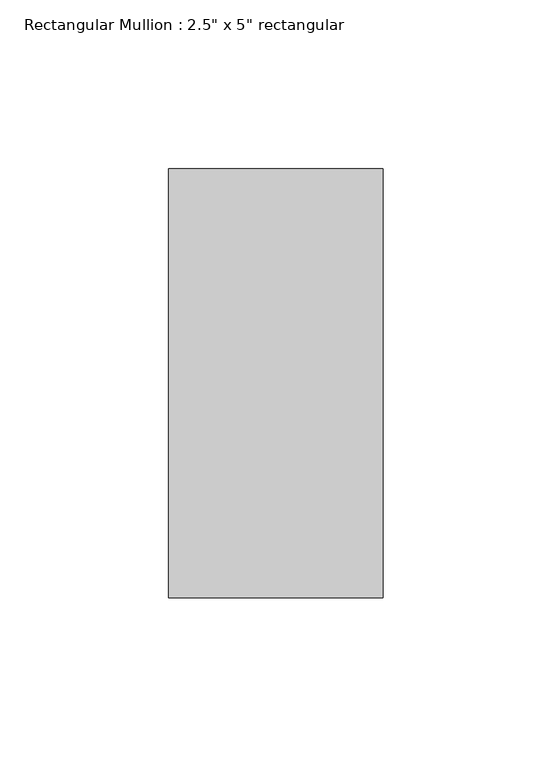
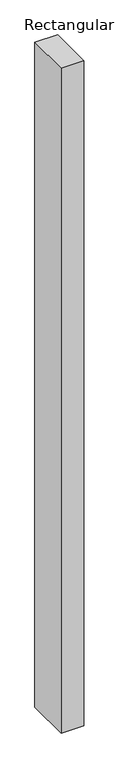
"""IFC4 building model written with IfcOpenShell, lengths in millimetres: member geometry."""

from ifc_helpers import new_model, si_unit, frame, origin, place, context, project, spatial, polyline, outline, extrude, source, transform, mapped, element, save


def member_1f3b6741(model_context):
    return source(origin(), model_context, "Body", "SweptSolid", [
        extrude(outline(polyline([(31.75, 63.5), (31.75, -63.5), (-31.75, -63.5), (-31.75, 63.5), (31.75, 63.5)])), frame((0.0, 0.0, -1964.4891744), z_axis=(0.0, 0.0, 1.0), x_axis=(1.0, 0.0, 0.0)), (0.0, 0.0, 1.0), 1964.4891744),
    ])


if __name__ == "__main__":
    model = new_model("IFC4")
    model_context = context("Model", 3, world=origin())
    ifc_project = project(units=[si_unit("LENGTHUNIT", "METRE", prefix="MILLI")], contexts=[model_context])
    site = spatial("IfcSite", under=ifc_project)
    building = spatial("IfcBuilding", under=site)
    placement = place(None, origin())
    member_shape = member_1f3b6741(model_context)
    element("IfcMember", 1, ObjectType="Rectangular Mullion : 2.5\" x 5\" rectangular", at=placement, inside=building, context=model_context, shape_type="MappedRepresentation", body=[
        mapped(member_shape, transform((0.0, 0.0, 0.0), x_axis=(1.0, 0.0, 0.0), y_axis=(0.0, 1.0, 0.0), z_axis=(0.0, 0.0, 1.0))),
    ])
    save(model, "model.ifc")

# Revit data of these elements
# Type "Rectangular Mullion : 2.5\" x 5\" rectangular"
#   built-in parameter 1007304 = 0.416667 (stored number, unit not read)
#   built-in parameter 1007301 = 0.104167 (stored number, unit not read)
#   built-in parameter 1007300 = 0.104167 (stored number, unit not read)
# Element 1 (IfcMember, "Rectangular Mullion : 2.5\" x 5\" rectangular")
#   Materials on its faces: "Aluminum"
# Materials
#   "Aluminum": class "Metal", colour RGB 247 247 247, transparency 0, Description = "Aluminum 6061", Cost = 0
